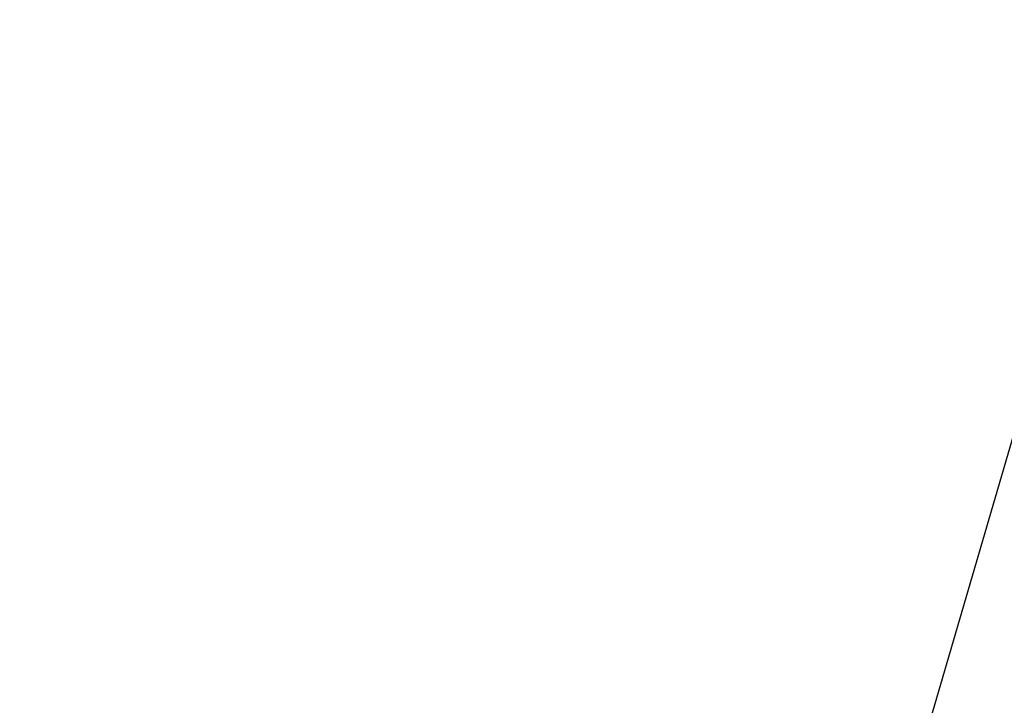
# Model space of a CAD drawing. Units: inches. Extents: x 3590 to 5167, y 65 to 1917.
# Tile 91 of 100: x 5052.5773 to 5052.8768, y 1788.8231 to 1789.0318. Entities that reach past the tile are written whole.
import ezdxf

# ---------------------------------------------------------------- set-up
doc = ezdxf.new("R2010")
doc.units = ezdxf.units.IN
for name, color, linetype, lineweight in [('A-ANNO-DIMS', 2, 'Continuous', 18), ('A-FLOR-PATT', 8, 'Continuous', 13), ('L-PLNT', 94, 'Continuous', 18)]:
    doc.layers.add(name, color=color, linetype=linetype, lineweight=lineweight)
doc.layers.add('DIENHOA', color=3, linetype='Continuous')
doc.styles.get("Standard").update_dxf_attribs({"font": 'arial.ttf'})
doc.dimstyles.new('ISO-25', dxfattribs={"dimtxt": 9, "dimasz": 2.5, "dimexe": 1.25, "dimexo": 0.625, "dimtad": 1, "dimdec": 1, "dimlunit": 3, "dimtxsty": 'Standard', "dimcen": 2.5, "dimadec": 0, "dimazin": 0, "dimtfac": 1, "dimtdec": 1, "dimtmove": 0, "dimatfit": 3, "dimfxl": 1, "dimarcsym": 0})

# ---------------------------------------------------------------- blocks, each defined once
blk = doc.blocks.new('Cay03_mb')
at = {"layer": 'DIENHOA'}
blk.add_line((118.956, 441.661), (96.72, 365.576), dxfattribs=at)
blk = doc.blocks.new('*D323')
at = {"layer": 'A-ANNO-DIMS', "color": 0, "lineweight": -2, "transparency": 16777216}
for p, q in [((5069.17227, 1795.21603), (5069.17227, 1874.95034)), ((5065.43703, 1795.21603), (5070.42227, 1795.21603)), ((5069.17227, 1769.30924), (5069.17227, 1792.71603)), ((5065.43703, 1766.80924), (5070.42227, 1766.80924))]:
    blk.add_line(p, q, dxfattribs=at)
at = {"layer": 'A-ANNO-DIMS', "color": 0, "transparency": 16777216}
for points in [[(5068.75561, 1792.71603), (5069.58894, 1792.71603), (5069.17227, 1795.21603)], [(5068.75561, 1769.30924), (5069.58894, 1769.30924), (5069.17227, 1766.80924)]]:
    blk.add_solid(points, dxfattribs=at)
at = {"layer": 'Defpoints', "color": 0, "transparency": 16777216}
for p in [(5064.81203, 1795.21603), (5069.17227, 1795.21603), (5064.81203, 1766.80924)]:
    blk.add_point(p, dxfattribs=at)
at = {"layer": 'A-ANNO-DIMS', "color": 0, "transparency": 16777216, "insert": (5063.89379, 1836.33318), "char_height": 9, "attachment_point": 5, "rotation": 90}
blk.add_mtext('2\'-4 1/2" TYP.', dxfattribs=at)

msp = doc.modelspace()

# ---------------------------------------------------------------- hatches: boundary and pattern name
at = {"layer": 'A-FLOR-PATT', "transparency": 33554687}
h = msp.add_hatch(dxfattribs=at)
h.set_pattern_fill('AR-HBONE', color=256, scale=0.2)
h.set_pattern_definition([(45, (-588.972, 0), (0, 28.73682), [60.96, -20.32]), (135, (-574.604, 14.368), (3e-15, 28.73682), [60.96, -20.32])])
h.paths.add_polyline_path([(5071.27403, 1796.99898), (4933.27403, 1796.99898), (4933.27403, 1753.99898), (4962.77403, 1753.99898, -0.414214), (4928.77403, 1719.99898), (4933.27403, 1718.99898), (4933.27403, 1334.99898), (5071.27403, 1334.99898)])
h.paths.add_polyline_path([(4951.78002, 1521.0767), (4951.7151, 1521.0404), (4951.56345, 1520.89532)], flags=16)
h.paths.add_polyline_path([(4952.267, 1521.37645), (4952.1977, 1521.37111), (4952.19823, 1521.35558)], flags=0)
h.paths.add_polyline_path([(4967.05076, 1529.72832), (4965.23122, 1528.69444), (4963.41109, 1527.71401), (4961.75649, 1526.85081), (4963.58887, 1527.44938), (4964.03555, 1527.47802), (4962.9755, 1527.24902), (4961.76022, 1526.85203), (4959.79219, 1525.83406), (4958.00498, 1524.89483), (4956.24031, 1523.92961), (4954.50395, 1522.91854), (4954.1294, 1522.68163), (4953.36051, 1521.99688), (4953.36558, 1521.99754), (4953.605, 1522.06367), (4955.10605, 1522.76083), (4956.92108, 1523.43405), (4958.67784, 1523.91513), (4960.35834, 1524.20036), (4961.94456, 1524.28606), (4964.17144, 1524.10849), (4965.95752, 1523.30903), (4963.86273, 1522.97565), (4965.18742, 1522.49898), (4963.36614, 1522.49715), (4961.54526, 1522.48682), (4959.76359, 1522.46077), (4958.30414, 1522.4188), (4957.97356, 1522.38829), (4956.30692, 1522.2324), (4954.71821, 1522.07143), (4953.25077, 1521.89915), (4953.52509, 1521.62277), (4954.33087, 1521.37883), (4956.24263, 1521.22987), (4958.03913, 1520.92952), (4959.68424, 1520.48339), (4961.16007, 1519.89569), (4963.10699, 1518.80022), (4964.39286, 1517.32518), (4962.97306, 1517.72596), (4964.55841, 1516.66059), (4965.40664, 1515.70779), (4963.50733, 1516.32179), (4961.67995, 1517.0051), (4959.93478, 1517.74489), (4958.2821, 1518.52833), (4956.73216, 1519.34257), (4955.29527, 1520.17478), (4954.67155, 1520.57237), (4954.51279, 1520.6271), (4955.65848, 1519.31837), (4956.70263, 1517.98232), (4957.64403, 1516.64663), (4958.48545, 1515.33439), (4959.54998, 1513.52398), (4960.43768, 1511.76936), (4958.84107, 1513.6196), (4957.45175, 1515.3249), (4955.8186, 1517.45855), (4956.66537, 1515.44764), (4957.11109, 1513.92292), (4957.44681, 1511.71434), (4957.07641, 1509.79288), (4956.53757, 1511.1103), (4955.99231, 1512.56892), (4955.44448, 1514.12509), (4954.89794, 1515.73518), (4954.35653, 1517.35553), (4953.82412, 1518.94251), (4953.30455, 1520.45247), (4953.06452, 1521.11563), (4952.97143, 1521.14607), (4952.94932, 1521.08646), (4952.72981, 1520.19905), (4953.3698, 1518.02364), (4953.75708, 1516.37279), (4954.05124, 1514.76538), (4954.26449, 1513.22121), (4954.47124, 1511.13121), (4954.4971, 1510.40174), (4954.40903, 1511.76006), (4954.26449, 1513.22121), (4954.05124, 1514.76538), (4953.75708, 1516.37279), (4953.3698, 1518.02364), (4952.87718, 1519.69813), (4952.7161, 1520.1412), (4952.53301, 1519.05871), (4952.37428, 1517.78881), (4952.21925, 1516.31167), (4952.04598, 1514.59986), (4951.83253, 1512.62598), (4951.55697, 1510.36259), (4951.20331, 1512.16818), (4950.85168, 1514.33931), (4950.98529, 1516.37594), (4951.6596, 1518.28625), (4952.59261, 1520.48085), (4952.35664, 1521.1299), (4951.85502, 1520.32753), (4950.83901, 1518.90828), (4949.77675, 1517.58658), (4948.91554, 1516.61731), (4948.11099, 1515.2561), (4947.0891, 1513.55389), (4945.88937, 1511.61495), (4946.32587, 1513.40232), (4946.5624, 1514.24913), (4945.52771, 1513.32668), (4944.58105, 1512.53126), (4946.01774, 1514.50825), (4947.2044, 1516.04763), (4947.89331, 1517.31331), (4949.30686, 1518.76446), (4950.41417, 1519.76716), (4950.45131, 1519.80628), (4952.267, 1521.37645), (4951.64457, 1521.49317), (4950.40371, 1521.17954), (4948.04447, 1520.35868), (4946.11863, 1519.45198), (4944.57182, 1518.47484), (4943.34962, 1517.44265), (4941.99695, 1515.91971), (4941.66146, 1515.27475), (4942.81332, 1516.98973), (4944.57182, 1518.47484), (4946.11863, 1519.45198), (4948.04447, 1520.35868), (4950.40371, 1521.17954), (4951.64457, 1521.49317), (4949.64678, 1521.86781), (4948.59979, 1521.75633), (4947.12629, 1521.5699), (4945.42015, 1521.34763), (4943.44969, 1521.10462), (4941.18319, 1520.85596), (4942.86028, 1521.61265), (4943.87308, 1522.03014), (4942.95216, 1521.9093), (4941.40968, 1521.48512), (4939.54287, 1520.67019), (4938.96775, 1520.2255), (4940.73284, 1521.29899), (4942.95216, 1521.9093), (4943.70184, 1522.00767), (4945.89419, 1522.69998), (4947.56488, 1522.71399), (4948.92086, 1522.56573), (4951.13144, 1522.18271), (4950.97062, 1522.2969), (4948.12924, 1523.00563), (4946.03496, 1523.70671), (4944.23235, 1524.52143), (4942.70692, 1525.46111), (4941.44419, 1526.53707), (4940.42968, 1527.76062), (4939.6489, 1529.14306), (4941.42091, 1528.12232), (4943.14742, 1527.13248), (4944.84093, 1526.17457), (4946.51394, 1525.24959), (4948.17893, 1524.35855), (4948.36457, 1524.26336), (4946.47531, 1526.04459), (4945.18083, 1527.54042), (4944.19039, 1529.03339), (4943.49559, 1530.53985), (4943.27808, 1531.3597), (4942.49849, 1531.91903), (4943.11353, 1531.76249), (4942.95927, 1533.6586), (4944.13953, 1531.9886), (4944.61171, 1531.32339), (4946.20163, 1530.46341), (4947.48567, 1529.50925), (4948.79027, 1528.22649), (4950.36754, 1526.23746), (4949.48547, 1528.15549), (4948.85128, 1530.12254), (4948.49054, 1532.04127), (4948.38105, 1533.91822), (4948.50062, 1535.7599), (4948.82704, 1537.57284), (4949.41803, 1535.56526), (4949.95684, 1533.56932), (4950.46414, 1531.5861), (4950.96058, 1529.6167), (4951.3911, 1527.95448), (4951.72352, 1530.68689), (4952.20106, 1532.57994), (4952.88914, 1534.32964), (4953.77035, 1535.95123), (4954.82726, 1537.45995), (4954.52145, 1535.38966), (4954.27314, 1533.93684), (4955.57999, 1535.6627), (4956.74758, 1536.73859), (4956.15852, 1534.78029), (4955.58917, 1532.87334), (4955.04336, 1531.00581), (4954.52493, 1529.16576), (4954.03771, 1527.34127), (4953.63833, 1525.73298), (4953.61143, 1525.58564), (4953.39805, 1524.16565), (4953.38219, 1524.00887), (4954.06955, 1525.47563), (4954.91212, 1527.02173), (4956.13627, 1528.89351), (4957.84668, 1530.57701), (4959.37601, 1531.54014), (4958.25596, 1530.10398), (4957.14284, 1528.66291), (4956.06626, 1527.24305), (4955.05579, 1525.87054), (4954.14104, 1524.57149), (4953.35159, 1523.37204), (4953.31079, 1523.30299), (4953.27253, 1522.92478), (4953.26102, 1522.38213), (4954.1031, 1523.37273), (4954.63005, 1524.28376), (4955.96149, 1526.35767), (4957.23002, 1528.12969), (4958.42057, 1529.60864), (4960.03671, 1531.36792), (4961.3736, 1532.3752), (4962.1015, 1532.77), (4961.06994, 1531.06113), (4959.98733, 1529.43811), (4958.86851, 1527.90803), (4958.15046, 1527.00742), (4959.80291, 1528.00314), (4961.58854, 1528.79257), (4963.39087, 1529.32783), (4965.21118, 1529.63205)], flags=16)
h.paths.add_polyline_path([(4962.94387, 1523.18187), (4961.10714, 1523.42192), (4960.39205, 1523.36158), (4962.34964, 1523.33061)], flags=0)
h.paths.add_polyline_path([(5049.54129, 1584.55089), (5049.47636, 1584.51458), (5049.32471, 1584.3695)], flags=16)
h.paths.add_polyline_path([(5050.02827, 1584.85063), (5049.95897, 1584.84529), (5049.95949, 1584.82976)], flags=0)
h.paths.add_polyline_path([(5042.33308, 1581.94902), (5043.8799, 1582.92616), (5045.80573, 1583.83286), (5048.16498, 1584.65372), (5049.40583, 1584.96736), (5047.40804, 1585.34199), (5046.36106, 1585.23052), (5044.88755, 1585.04408), (5043.18142, 1584.82181), (5041.21095, 1584.5788), (5038.94446, 1584.33014), (5040.62155, 1585.08683), (5041.63434, 1585.50432), (5040.71343, 1585.38348), (5039.17095, 1584.9593), (5037.30414, 1584.14438), (5036.72901, 1583.69969), (5038.4941, 1584.77317), (5040.71343, 1585.38348), (5041.4631, 1585.48185), (5043.65545, 1586.17416), (5045.32615, 1586.18818), (5046.68212, 1586.03992), (5048.8927, 1585.6569), (5048.73188, 1585.77108), (5045.89051, 1586.47981), (5043.79622, 1587.18089), (5041.99361, 1587.99561), (5040.46818, 1588.9353), (5039.20546, 1590.01125), (5038.19095, 1591.2348), (5037.41016, 1592.61725), (5039.18217, 1591.5965), (5040.90868, 1590.60667), (5042.6022, 1589.64876), (5044.2752, 1588.72378), (5045.94019, 1587.83274), (5046.12584, 1587.73754), (5044.23658, 1589.51878), (5042.9421, 1591.01461), (5041.95166, 1592.50757), (5041.25685, 1594.01403), (5041.03935, 1594.83388), (5040.25976, 1595.39321), (5040.8748, 1595.23667), (5040.72054, 1597.13279), (5041.9008, 1595.46278), (5042.37297, 1594.79758), (5043.96289, 1593.93759), (5045.24694, 1592.98344), (5046.55153, 1591.70068), (5048.12881, 1589.71164), (5047.24673, 1591.62967), (5046.61254, 1593.59672), (5046.2518, 1595.51546), (5046.14232, 1597.3924), (5046.26189, 1599.23408), (5046.5883, 1601.04703), (5047.17929, 1599.03944), (5047.71811, 1597.0435), (5048.22541, 1595.06028), (5048.72184, 1593.09089), (5049.15237, 1591.42866), (5049.48478, 1594.16107), (5049.96233, 1596.05412), (5050.65041, 1597.80382), (5051.53161, 1599.42541), (5052.58852, 1600.93414), (5052.28271, 1598.86384), (5052.03441, 1597.41102), (5053.34126, 1599.13689), (5054.50884, 1600.21277), (5053.91979, 1598.25447), (5053.35044, 1596.34752), (5052.80463, 1594.47999), (5052.2862, 1592.63995), (5051.79898, 1590.81546), (5051.39959, 1589.20716), (5051.3727, 1589.05983), (5051.15931, 1587.63984), (5051.14346, 1587.48305), (5051.83082, 1588.94982), (5052.67339, 1590.49592), (5053.89754, 1592.3677), (5055.60794, 1594.05119), (5057.13728, 1595.01432), (5056.01722, 1593.57817), (5054.90411, 1592.1371), (5053.82752, 1590.71724), (5052.81705, 1589.34472), (5051.9023, 1588.04567), (5051.11286, 1586.84622), (5051.07205, 1586.77718), (5051.03379, 1586.39896), (5051.02228, 1585.85631), (5051.86437, 1586.84692), (5052.39131, 1587.75794), (5053.72275, 1589.83185), (5054.99128, 1591.60387), (5056.18183, 1593.08282), (5057.79798, 1594.84211), (5059.13486, 1595.84938), (5059.86276, 1596.24419), (5058.83121, 1594.53531), (5057.7486, 1592.9123), (5056.62978, 1591.38221), (5055.91173, 1590.4816), (5057.56418, 1591.47732), (5059.34981, 1592.26675), (5061.15214, 1592.80202), (5062.97245, 1593.10624), (5064.81203, 1593.20251), (5062.99248, 1592.16863), (5061.17235, 1591.18819), (5059.51775, 1590.325), (5061.35014, 1590.92356), (5061.79682, 1590.95221), (5060.73676, 1590.7232), (5059.52148, 1590.32622), (5057.55345, 1589.30825), (5055.76625, 1588.36901), (5054.00157, 1587.40379), (5052.26521, 1586.39273), (5051.89067, 1586.15581), (5051.12177, 1585.47106), (5051.12684, 1585.47172), (5051.36627, 1585.53786), (5052.86732, 1586.23502), (5054.68234, 1586.90824), (5056.4391, 1587.38931), (5058.1196, 1587.67454), (5059.70582, 1587.76024), (5061.93271, 1587.58268), (5063.71878, 1586.78321), (5061.62399, 1586.44983), (5062.94869, 1585.97317), (5061.12741, 1585.97133), (5059.30653, 1585.961), (5057.52486, 1585.93496), (5056.06541, 1585.89299), (5055.73482, 1585.86247), (5054.06819, 1585.70658), (5052.47947, 1585.54561), (5051.01204, 1585.37333), (5051.28635, 1585.09695), (5052.09214, 1584.85301), (5054.00389, 1584.70406), (5055.8004, 1584.4037), (5057.44551, 1583.95757), (5058.92133, 1583.36987), (5060.86825, 1582.27441), (5062.15413, 1580.79937), (5060.73433, 1581.20015), (5062.31967, 1580.13477), (5063.1679, 1579.18198), (5061.2686, 1579.79597), (5059.44122, 1580.47928), (5057.69605, 1581.21908), (5056.04336, 1582.00251), (5054.49343, 1582.81675), (5053.05653, 1583.64897), (5052.43281, 1584.04656), (5052.27405, 1584.10128), (5053.41974, 1582.79255), (5054.4639, 1581.4565), (5055.40529, 1580.12081), (5056.24672, 1578.80858), (5057.31125, 1576.99816), (5058.19895, 1575.24354), (5056.60234, 1577.09378), (5055.21301, 1578.79908), (5053.57987, 1580.93274), (5054.42664, 1578.92183), (5054.87235, 1577.3971), (5055.20808, 1575.18852), (5054.83767, 1573.26706), (5054.29883, 1574.58448), (5053.75357, 1576.0431), (5053.20575, 1577.59927), (5052.6592, 1579.20936), (5052.1178, 1580.82971), (5051.58538, 1582.41669), (5051.06582, 1583.92666), (5050.82578, 1584.58981), (5050.7327, 1584.62025), (5050.71058, 1584.56064), (5050.49108, 1583.67323), (5051.13107, 1581.49782), (5051.51835, 1579.84698), (5051.8125, 1578.23957), (5052.02575, 1576.69539), (5052.23251, 1574.6054), (5052.25836, 1573.87593), (5052.1703, 1575.23424), (5052.02575, 1576.69539), (5051.8125, 1578.23957), (5051.51835, 1579.84698), (5051.13107, 1581.49782), (5050.63844, 1583.17231), (5050.47736, 1583.61538), (5050.29428, 1582.53289), (5050.13554, 1581.26299), (5049.98051, 1579.78585), (5049.80724, 1578.07405), (5049.59379, 1576.10016), (5049.31823, 1573.83678), (5048.96458, 1575.64237), (5048.61294, 1577.8135), (5048.74656, 1579.85012), (5049.42086, 1581.76043), (5050.35388, 1583.95503), (5050.1179, 1584.60408), (5049.61629, 1583.80172), (5048.60027, 1582.38246), (5047.53801, 1581.06076), (5046.67681, 1580.09149), (5045.87225, 1578.73029), (5044.85036, 1577.02808), (5043.65063, 1575.08913), (5044.08713, 1576.8765), (5044.32366, 1577.72331), (5043.28898, 1576.80086), (5042.34232, 1576.00545), (5043.779, 1577.98243), (5044.96566, 1579.52182), (5045.65457, 1580.78749), (5047.06813, 1582.23865), (5048.17543, 1583.24134), (5048.21258, 1583.28047), (5050.02827, 1584.85063), (5049.40583, 1584.96736), (5048.16498, 1584.65372), (5045.80573, 1583.83286), (5043.8799, 1582.92616), (5042.33308, 1581.94902), (5041.11088, 1580.91684), (5039.75821, 1579.39389), (5039.42272, 1578.74894), (5040.57458, 1580.46391)], flags=16)
h.paths.add_polyline_path([(4954.79872, 1533.12029), (4954.26249, 1532.07935), (4953.83112, 1530.93464), (4953.50472, 1529.63602), (4953.28338, 1528.13331), (4953.16721, 1526.37637), (4953.15631, 1524.31504), (4953.27669, 1521.23629), (4952.80168, 1521.84177), (4951.55695, 1521.99789), (4950.97575, 1521.9613), (4952.66059, 1521.94097), (4952.80168, 1521.84177), (4953.15249, 1523.59258), (4953.16721, 1526.37637), (4953.28338, 1528.13331), (4953.60929, 1530.34598), (4954.45558, 1532.59174)], flags=0)
h.paths.add_polyline_path([(5050.56294, 1585.31596), (5049.31822, 1585.47208), (5048.73702, 1585.43548), (5050.42186, 1585.41516), (5050.56294, 1585.31596), (5050.91375, 1587.06676), (5050.92848, 1589.85056), (5051.04465, 1591.6075), (5051.37055, 1593.82017), (5052.21684, 1596.06593), (5052.55999, 1596.59447), (5052.02375, 1595.55353), (5051.59238, 1594.40883), (5051.26598, 1593.1102), (5051.04465, 1591.6075), (5050.92848, 1589.85056), (5050.91757, 1587.78922), (5051.03795, 1584.71048)], flags=0)
h.paths.add_polyline_path([(5058.15332, 1586.83576), (5060.11091, 1586.80479), (5060.70514, 1586.65605), (5058.8684, 1586.8961)], flags=0)
h.paths.add_polyline_path([(5049.54129, 1430.93611), (5049.47636, 1430.8998), (5049.32471, 1430.75472)], flags=16)
h.paths.add_polyline_path([(5050.02827, 1431.23585), (5049.95897, 1431.23051), (5049.95949, 1431.21498)], flags=0)
h.paths.add_polyline_path([(5046.5883, 1447.43225), (5047.17929, 1445.42467), (5047.71811, 1443.42872), (5048.22541, 1441.4455), (5048.72184, 1439.47611), (5049.15237, 1437.81388), (5049.48478, 1440.5463), (5049.96233, 1442.43934), (5050.65041, 1444.18904), (5051.53161, 1445.81063), (5052.58852, 1447.31936), (5052.28271, 1445.24906), (5052.03441, 1443.79624), (5053.34126, 1445.52211), (5054.50884, 1446.59799), (5053.91979, 1444.63969), (5053.35044, 1442.73274), (5052.80463, 1440.86521), (5052.2862, 1439.02517), (5051.79898, 1437.20068), (5051.39959, 1435.59238), (5051.3727, 1435.44505), (5051.15931, 1434.02506), (5051.14346, 1433.86828), (5051.83082, 1435.33504), (5052.67339, 1436.88114), (5053.89754, 1438.75292), (5055.60794, 1440.43641), (5057.13728, 1441.39954), (5056.01722, 1439.96339), (5054.90411, 1438.52232), (5053.82752, 1437.10246), (5052.81705, 1435.72994), (5051.9023, 1434.4309), (5051.11286, 1433.23145), (5051.07205, 1433.1624), (5051.03379, 1432.78418), (5051.02228, 1432.24153), (5051.86437, 1433.23214), (5052.39131, 1434.14316), (5053.72275, 1436.21707), (5054.99128, 1437.98909), (5056.18183, 1439.46805), (5057.79798, 1441.22733), (5059.13486, 1442.23461), (5059.86276, 1442.62941), (5058.83121, 1440.92053), (5057.7486, 1439.29752), (5056.62978, 1437.76743), (5055.91173, 1436.86682), (5057.56418, 1437.86255), (5059.34981, 1438.65197), (5061.15214, 1439.18724), (5062.97245, 1439.49146), (5064.81203, 1439.58773), (5062.99248, 1438.55385), (5061.17235, 1437.57342), (5059.51775, 1436.71022), (5061.35014, 1437.30879), (5061.79682, 1437.33743), (5060.73676, 1437.10842), (5059.52148, 1436.71144), (5057.55345, 1435.69347), (5055.76625, 1434.75423), (5054.00157, 1433.78901), (5052.26521, 1432.77795), (5051.89067, 1432.54103), (5051.12177, 1431.85628), (5051.12684, 1431.85694), (5051.36627, 1431.92308), (5052.86732, 1432.62024), (5054.68234, 1433.29346), (5056.4391, 1433.77453), (5058.1196, 1434.05976), (5059.70582, 1434.14546), (5061.93271, 1433.9679), (5063.71878, 1433.16843), (5061.62399, 1432.83505), (5062.94869, 1432.35839), (5061.12741, 1432.35655), (5059.30653, 1432.34623), (5057.52486, 1432.32018), (5056.06541, 1432.27821), (5055.73482, 1432.24769), (5054.06819, 1432.09181), (5052.47947, 1431.93083), (5051.01204, 1431.75856), (5051.28635, 1431.48218), (5052.09214, 1431.23823), (5054.00389, 1431.08928), (5055.8004, 1430.78892), (5057.44551, 1430.34279), (5058.92133, 1429.75509), (5060.86825, 1428.65963), (5062.15413, 1427.18459), (5060.73433, 1427.58537), (5062.31967, 1426.52), (5063.1679, 1425.5672), (5061.2686, 1426.18119), (5059.44122, 1426.86451), (5057.69605, 1427.6043), (5056.04336, 1428.38773), (5054.49343, 1429.20197), (5053.05653, 1430.03419), (5052.43281, 1430.43178), (5052.27405, 1430.48651), (5053.41974, 1429.17777), (5054.4639, 1427.84172), (5055.40529, 1426.50603), (5056.24672, 1425.1938), (5057.31125, 1423.38338), (5058.19895, 1421.62877), (5056.60234, 1423.479), (5055.21301, 1425.1843), (5053.57987, 1427.31796), (5054.42664, 1425.30705), (5054.87235, 1423.78233), (5055.20808, 1421.57374), (5054.83767, 1419.65228), (5054.29883, 1420.9697), (5053.75357, 1422.42832), (5053.20575, 1423.9845), (5052.6592, 1425.59458), (5052.1178, 1427.21493), (5051.58538, 1428.80191), (5051.06582, 1430.31188), (5050.82578, 1430.97503), (5050.7327, 1431.00547), (5050.71058, 1430.94586), (5050.49108, 1430.05845), (5051.13107, 1427.88305), (5051.51835, 1426.2322), (5051.8125, 1424.62479), (5052.02575, 1423.08061), (5052.23251, 1420.99062), (5052.25836, 1420.26115), (5052.1703, 1421.61947), (5052.02575, 1423.08061), (5051.8125, 1424.62479), (5051.51835, 1426.2322), (5051.13107, 1427.88305), (5050.63844, 1429.55753), (5050.47736, 1430.0006), (5050.29428, 1428.91811), (5050.13554, 1427.64821), (5049.98051, 1426.17107), (5049.80724, 1424.45927), (5049.59379, 1422.48539), (5049.31823, 1420.222), (5048.96458, 1422.02759), (5048.61294, 1424.19872), (5048.74656, 1426.23534), (5049.42086, 1428.14565), (5050.35388, 1430.34025), (5050.1179, 1430.98931), (5049.61629, 1430.18694), (5048.60027, 1428.76768), (5047.53801, 1427.44598), (5046.67681, 1426.47671), (5045.87225, 1425.11551), (5044.85036, 1423.4133), (5043.65063, 1421.47435), (5044.08713, 1423.26172), (5044.32366, 1424.10854), (5043.28898, 1423.18608), (5042.34232, 1422.39067), (5043.779, 1424.36765), (5044.96566, 1425.90704), (5045.65457, 1427.17272), (5047.06813, 1428.62387), (5048.17543, 1429.62657), (5048.21258, 1429.66569), (5050.02827, 1431.23585), (5049.40583, 1431.35258), (5048.16498, 1431.03894), (5045.80573, 1430.21809), (5043.8799, 1429.31139), (5042.33308, 1428.33424), (5041.11088, 1427.30206), (5039.75821, 1425.77911), (5039.42272, 1425.13416), (5040.57458, 1426.84914), (5042.33308, 1428.33424), (5043.8799, 1429.31139), (5045.80573, 1430.21809), (5048.16498, 1431.03894), (5049.40583, 1431.35258), (5047.40804, 1431.72722), (5046.36106, 1431.61574), (5044.88755, 1431.42931), (5043.18142, 1431.20704), (5041.21095, 1430.96402), (5038.94446, 1430.71536), (5040.62155, 1431.47205), (5041.63434, 1431.88954), (5040.71343, 1431.76871), (5039.17095, 1431.34453), (5037.30414, 1430.5296), (5036.72901, 1430.08491), (5038.4941, 1431.1584), (5040.71343, 1431.76871), (5041.4631, 1431.86707), (5043.65545, 1432.55939), (5045.32615, 1432.5734), (5046.68212, 1432.42514), (5048.8927, 1432.04212), (5048.73188, 1432.1563), (5045.89051, 1432.86503), (5043.79622, 1433.56611), (5041.99361, 1434.38083), (5040.46818, 1435.32052), (5039.20546, 1436.39648), (5038.19095, 1437.62002), (5037.41016, 1439.00247), (5039.18217, 1437.98172), (5040.90868, 1436.99189), (5042.6022, 1436.03398), (5044.2752, 1435.109), (5045.94019, 1434.21796), (5046.12584, 1434.12276), (5044.23658, 1435.904), (5042.9421, 1437.39983), (5041.95166, 1438.8928), (5041.25685, 1440.39925), (5041.03935, 1441.2191), (5040.25976, 1441.77844), (5040.8748, 1441.62189), (5040.72054, 1443.51801), (5041.9008, 1441.848), (5042.37297, 1441.1828), (5043.96289, 1440.32282), (5045.24694, 1439.36866), (5046.55153, 1438.0859), (5048.12881, 1436.09686), (5047.24673, 1438.01489), (5046.61254, 1439.98195), (5046.2518, 1441.90068), (5046.14232, 1443.77762), (5046.26189, 1445.6193)], flags=16)
h.paths.add_polyline_path([(5052.38176, 1444.25496), (5051.62263, 1442.77987), (5052.02375, 1441.93875), (5052.55999, 1442.9797)], flags=0)
h.paths.add_polyline_path([(5050.56294, 1431.70118), (5049.31822, 1431.8573), (5048.73702, 1431.82071), (5050.42186, 1431.80038)], flags=0)
h.paths.add_polyline_path([(5058.15332, 1433.22098), (5060.11091, 1433.19001), (5060.70514, 1433.04127), (5058.8684, 1433.28132)], flags=0)
h.paths.add_polyline_path([(5049.54129, 1352.28535), (5049.47636, 1352.24904), (5049.32471, 1352.10396)], flags=16)
h.paths.add_polyline_path([(5050.02827, 1352.58509), (5049.95897, 1352.57975), (5049.95949, 1352.56422)], flags=0)
h.paths.add_polyline_path([(5046.5883, 1368.78149), (5047.17929, 1366.7739), (5047.71811, 1364.77796), (5048.22541, 1362.79474), (5048.72184, 1360.82534), (5049.15237, 1359.16312), (5049.48478, 1361.89553), (5049.96233, 1363.78858), (5050.65041, 1365.53828), (5051.53161, 1367.15987), (5052.58852, 1368.6686), (5052.28271, 1366.5983), (5052.03441, 1365.14548), (5053.34126, 1366.87135), (5054.50884, 1367.94723), (5053.91979, 1365.98893), (5053.35044, 1364.08198), (5052.80463, 1362.21445), (5052.2862, 1360.37441), (5051.79898, 1358.54992), (5051.39959, 1356.94162), (5051.3727, 1356.79428), (5051.15931, 1355.37429), (5051.14346, 1355.21751), (5051.83082, 1356.68428), (5052.67339, 1358.23037), (5053.89754, 1360.10216), (5055.60794, 1361.78565), (5057.13728, 1362.74878), (5056.01722, 1361.31262), (5054.90411, 1359.87155), (5053.82752, 1358.4517), (5052.81705, 1357.07918), (5051.9023, 1355.78013), (5051.11286, 1354.58068), (5051.07205, 1354.51164), (5051.03379, 1354.13342), (5051.02228, 1353.59077), (5051.86437, 1354.58137), (5052.39131, 1355.4924), (5053.72275, 1357.56631), (5054.99128, 1359.33833), (5056.18183, 1360.81728), (5057.79798, 1362.57656), (5059.13486, 1363.58384), (5059.86276, 1363.97864), (5058.83121, 1362.26977), (5057.7486, 1360.64675), (5056.62978, 1359.11667), (5055.91173, 1358.21606), (5057.56418, 1359.21178), (5059.34981, 1360.00121), (5061.15214, 1360.53648), (5062.97245, 1360.84069), (5064.81203, 1360.93697), (5062.99248, 1359.90308), (5061.17235, 1358.92265), (5059.51775, 1358.05946), (5061.35014, 1358.65802), (5061.79682, 1358.68666), (5060.73676, 1358.45766), (5059.52148, 1358.06068), (5057.55345, 1357.0427), (5055.76625, 1356.10347), (5054.00157, 1355.13825), (5052.26521, 1354.12718), (5051.89067, 1353.89027), (5051.12177, 1353.20552), (5051.12684, 1353.20618), (5051.36627, 1353.27231), (5052.86732, 1353.96947), (5054.68234, 1354.6427), (5056.4391, 1355.12377), (5058.1196, 1355.409), (5059.70582, 1355.4947), (5061.93271, 1355.31713), (5063.71878, 1354.51767), (5061.62399, 1354.18429), (5062.94869, 1353.70763), (5061.12741, 1353.70579), (5059.30653, 1353.69546), (5057.52486, 1353.66942), (5056.06541, 1353.62744), (5055.73482, 1353.59693), (5054.06819, 1353.44104), (5052.47947, 1353.28007), (5051.01204, 1353.10779), (5051.28635, 1352.83141), (5052.09214, 1352.58747), (5054.00389, 1352.43852), (5055.8004, 1352.13816), (5057.44551, 1351.69203), (5058.92133, 1351.10433), (5060.86825, 1350.00887), (5062.15413, 1348.53382), (5060.73433, 1348.9346), (5062.31967, 1347.86923), (5063.1679, 1346.91643), (5061.2686, 1347.53043), (5059.44122, 1348.21374), (5057.69605, 1348.95353), (5056.04336, 1349.73697), (5054.49343, 1350.55121), (5053.05653, 1351.38342), (5052.43281, 1351.78101), (5052.27405, 1351.83574), (5053.41974, 1350.52701), (5054.4639, 1349.19096), (5055.40529, 1347.85527), (5056.24672, 1346.54303), (5057.31125, 1344.73262), (5058.19895, 1342.978), (5056.60234, 1344.82824), (5055.21301, 1346.53354), (5053.57987, 1348.6672), (5054.42664, 1346.65629), (5054.87235, 1345.13156), (5055.20808, 1342.92298), (5054.83767, 1341.00152), (5054.29883, 1342.31894), (5053.75357, 1343.77756), (5053.20575, 1345.33373), (5052.6592, 1346.94382), (5052.1178, 1348.56417), (5051.58538, 1350.15115), (5051.06582, 1351.66111), (5050.82578, 1352.32427), (5050.7327, 1352.35471), (5050.71058, 1352.2951), (5050.49108, 1351.40769), (5051.13107, 1349.23228), (5051.51835, 1347.58144), (5051.8125, 1345.97403), (5052.02575, 1344.42985), (5052.23251, 1342.33986), (5052.25836, 1341.61039), (5052.1703, 1342.9687), (5052.02575, 1344.42985), (5051.8125, 1345.97403), (5051.51835, 1347.58144), (5051.13107, 1349.23228), (5050.63844, 1350.90677), (5050.47736, 1351.34984), (5050.29428, 1350.26735), (5050.13554, 1348.99745), (5049.98051, 1347.52031), (5049.80724, 1345.80851), (5049.59379, 1343.83462), (5049.31823, 1341.57124), (5048.96458, 1343.37683), (5048.61294, 1345.54796), (5048.74656, 1347.58458), (5049.42086, 1349.49489), (5050.35388, 1351.68949), (5050.1179, 1352.33854), (5049.61629, 1351.53617), (5048.60027, 1350.11692), (5047.53801, 1348.79522), (5046.67681, 1347.82595), (5045.87225, 1346.46475), (5044.85036, 1344.76253), (5043.65063, 1342.82359), (5044.08713, 1344.61096), (5044.32366, 1345.45777), (5043.28898, 1344.53532), (5042.34232, 1343.7399), (5043.779, 1345.71689), (5044.96566, 1347.25627), (5045.65457, 1348.52195), (5047.06813, 1349.9731), (5048.17543, 1350.9758), (5048.21258, 1351.01493), (5050.02827, 1352.58509), (5049.40583, 1352.70181), (5048.16498, 1352.38818), (5045.80573, 1351.56732), (5043.8799, 1350.66062), (5042.33308, 1349.68348), (5041.11088, 1348.65129), (5039.75821, 1347.12835), (5039.42272, 1346.4834), (5040.57458, 1348.19837), (5042.33308, 1349.68348), (5043.8799, 1350.66062), (5045.80573, 1351.56732), (5048.16498, 1352.38818), (5049.40583, 1352.70181), (5047.40804, 1353.07645), (5046.36106, 1352.96498), (5044.88755, 1352.77854), (5043.18142, 1352.55627), (5041.21095, 1352.31326), (5038.94446, 1352.0646), (5040.62155, 1352.82129), (5041.63434, 1353.23878), (5040.71343, 1353.11794), (5039.17095, 1352.69376), (5037.30414, 1351.87884), (5036.72901, 1351.43415), (5038.4941, 1352.50763), (5040.71343, 1353.11794), (5041.4631, 1353.21631), (5043.65545, 1353.90862), (5045.32615, 1353.92263), (5046.68212, 1353.77438), (5048.8927, 1353.39136), (5048.73188, 1353.50554), (5045.89051, 1354.21427), (5043.79622, 1354.91535), (5041.99361, 1355.73007), (5040.46818, 1356.66975), (5039.20546, 1357.74571), (5038.19095, 1358.96926), (5037.41016, 1360.35171), (5039.18217, 1359.33096), (5040.90868, 1358.34112), (5042.6022, 1357.38321), (5044.2752, 1356.45824), (5045.94019, 1355.5672), (5046.12584, 1355.472), (5044.23658, 1357.25323), (5042.9421, 1358.74906), (5041.95166, 1360.24203), (5041.25685, 1361.74849), (5041.03935, 1362.56834), (5040.25976, 1363.12767), (5040.8748, 1362.97113), (5040.72054, 1364.86725), (5041.9008, 1363.19724), (5042.37297, 1362.53203), (5043.96289, 1361.67205), (5045.24694, 1360.7179), (5046.55153, 1359.43513), (5048.12881, 1357.4461), (5047.24673, 1359.36413), (5046.61254, 1361.33118), (5046.2518, 1363.24992), (5046.14232, 1365.12686), (5046.26189, 1366.96854)], flags=16)
h.paths.add_polyline_path([(5052.38176, 1365.6042), (5051.62263, 1364.12911), (5052.02375, 1363.28799), (5052.55999, 1364.32893)], flags=0)
h.paths.add_polyline_path([(4951.78002, 1698.04081), (4951.7151, 1698.0045), (4951.56345, 1697.85942)], flags=16)
h.paths.add_polyline_path([(4952.267, 1698.34055), (4952.1977, 1698.33521), (4952.19823, 1698.31968)], flags=0)
h.paths.add_polyline_path([(4957.07641, 1686.75698), (4956.53757, 1688.0744), (4955.99231, 1689.53302), (4955.44448, 1691.08919), (4954.89794, 1692.69928), (4954.35653, 1694.31963), (4953.82412, 1695.90661), (4953.30455, 1697.41658), (4953.06452, 1698.07973), (4952.97143, 1698.11017), (4952.94932, 1698.05056), (4952.72981, 1697.16315), (4953.3698, 1694.98774), (4953.75708, 1693.3369), (4954.05124, 1691.72949), (4954.26449, 1690.18531), (4954.47124, 1688.09532), (4954.4971, 1687.36585), (4954.40903, 1688.72416), (4954.26449, 1690.18531), (4954.05124, 1691.72949), (4953.75708, 1693.3369), (4953.3698, 1694.98774), (4952.87718, 1696.66223), (4952.7161, 1697.1053), (4952.53301, 1696.02281), (4952.37428, 1694.75291), (4952.21925, 1693.27577), (4952.04598, 1691.56397), (4951.83253, 1689.59008), (4951.55697, 1687.3267), (4951.20331, 1689.13229), (4950.85168, 1691.30342), (4950.98529, 1693.34004), (4951.6596, 1695.25035), (4952.59261, 1697.44495), (4952.35664, 1698.09401), (4951.85502, 1697.29164), (4950.83901, 1695.87238), (4949.77675, 1694.55068), (4948.91554, 1693.58141), (4948.11099, 1692.22021), (4947.0891, 1690.518), (4945.88937, 1688.57905), (4946.32587, 1690.36642), (4946.5624, 1691.21323), (4945.52771, 1690.29078), (4944.58105, 1689.49537), (4946.01774, 1691.47235), (4947.2044, 1693.01174), (4947.89331, 1694.27741), (4949.30686, 1695.72857), (4950.41417, 1696.73127), (4950.45131, 1696.77039), (4952.267, 1698.34055), (4951.64457, 1698.45728), (4950.40371, 1698.14364), (4948.04447, 1697.32278), (4946.11863, 1696.41608), (4944.57182, 1695.43894), (4943.34962, 1694.40676), (4941.99695, 1692.88381), (4941.66146, 1692.23886), (4942.81332, 1693.95383), (4944.57182, 1695.43894), (4946.11863, 1696.41608), (4948.04447, 1697.32278), (4950.40371, 1698.14364), (4951.64457, 1698.45728), (4949.64678, 1698.83191), (4948.59979, 1698.72044), (4947.12629, 1698.53401), (4945.42015, 1698.31174), (4943.44969, 1698.06872), (4941.18319, 1697.82006), (4942.86028, 1698.57675), (4943.87308, 1698.99424), (4942.95216, 1698.8734), (4941.40968, 1698.44922), (4939.54287, 1697.6343), (4938.96775, 1697.18961), (4940.73284, 1698.26309), (4942.95216, 1698.8734), (4943.70184, 1698.97177), (4945.89419, 1699.66409), (4947.56488, 1699.6781), (4948.92086, 1699.52984), (4951.13144, 1699.14682), (4950.97062, 1699.261), (4948.12924, 1699.96973), (4946.03496, 1700.67081), (4944.23235, 1701.48553), (4942.70692, 1702.42522), (4941.44419, 1703.50117), (4940.42968, 1704.72472), (4939.6489, 1706.10717), (4941.42091, 1705.08642), (4943.14742, 1704.09659), (4944.84093, 1703.13868), (4946.51394, 1702.2137), (4948.17893, 1701.32266), (4948.36457, 1701.22746), (4946.47531, 1703.0087), (4945.18083, 1704.50453), (4944.19039, 1705.9975), (4943.49559, 1707.50395), (4943.27808, 1708.3238), (4942.49849, 1708.88314), (4943.11353, 1708.72659), (4942.95927, 1710.62271), (4944.13953, 1708.9527), (4944.61171, 1708.2875), (4946.20163, 1707.42751), (4947.48567, 1706.47336), (4948.79027, 1705.1906), (4950.36754, 1703.20156), (4949.48547, 1705.11959), (4948.85128, 1707.08664), (4948.49054, 1709.00538), (4948.38105, 1710.88232), (4948.50062, 1712.724), (4948.82704, 1714.53695), (4949.41803, 1712.52937), (4949.95684, 1710.53342), (4950.46414, 1708.5502), (4950.96058, 1706.58081), (4951.3911, 1704.91858), (4951.72352, 1707.65099), (4952.20106, 1709.54404), (4952.88914, 1711.29374), (4953.77035, 1712.91533), (4954.82726, 1714.42406), (4954.52145, 1712.35376), (4954.27314, 1710.90094), (4955.57999, 1712.62681), (4956.74758, 1713.70269), (4956.15852, 1711.74439), (4955.58917, 1709.83744), (4955.04336, 1707.96991), (4954.52493, 1706.12987), (4954.03771, 1704.30538), (4953.63833, 1702.69708), (4953.61143, 1702.54975), (4953.39805, 1701.12976), (4953.38219, 1700.97297), (4954.06955, 1702.43974), (4954.91212, 1703.98584), (4956.13627, 1705.85762), (4957.84668, 1707.54111), (4959.37601, 1708.50424), (4958.25596, 1707.06809), (4957.14284, 1705.62702), (4956.06626, 1704.20716), (4955.05579, 1702.83464), (4954.14104, 1701.53559), (4953.35159, 1700.33614), (4953.31079, 1700.2671), (4953.27253, 1699.88888), (4953.26102, 1699.34623), (4954.1031, 1700.33684), (4954.63005, 1701.24786), (4955.96149, 1703.32177), (4957.23002, 1705.09379), (4958.42057, 1706.57274), (4960.03671, 1708.33203), (4961.3736, 1709.33931), (4962.1015, 1709.73411), (4961.06994, 1708.02523), (4959.98733, 1706.40222), (4958.86851, 1704.87213), (4958.15046, 1703.97152), (4959.80291, 1704.96725), (4961.58854, 1705.75667), (4963.39087, 1706.29194), (4965.21118, 1706.59616), (4967.05076, 1706.69243), (4965.23122, 1705.65855), (4963.41109, 1704.67811), (4961.75649, 1703.81492), (4963.58887, 1704.41349), (4964.03555, 1704.44213), (4962.9755, 1704.21312), (4961.76022, 1703.81614), (4959.79219, 1702.79817), (4958.00498, 1701.85893), (4956.24031, 1700.89371), (4954.50395, 1699.88265), (4954.1294, 1699.64573), (4953.36051, 1698.96098), (4953.36558, 1698.96164), (4953.605, 1699.02778), (4955.10605, 1699.72494), (4956.92108, 1700.39816), (4958.67784, 1700.87923), (4960.35834, 1701.16446), (4961.94456, 1701.25016), (4964.17144, 1701.0726), (4965.95752, 1700.27313), (4963.86273, 1699.93975), (4965.18742, 1699.46309), (4963.36614, 1699.46125), (4961.54526, 1699.45092), (4959.76359, 1699.42488), (4958.30414, 1699.38291), (4957.97356, 1699.35239), (4956.30692, 1699.1965), (4954.71821, 1699.03553), (4953.25077, 1698.86326), (4953.52509, 1698.58688), (4954.33087, 1698.34293), (4956.24263, 1698.19398), (4958.03913, 1697.89362), (4959.68424, 1697.44749), (4961.16007, 1696.85979), (4963.10699, 1695.76433), (4964.39286, 1694.28929), (4962.97306, 1694.69007), (4964.55841, 1693.6247), (4965.40664, 1692.6719), (4963.50733, 1693.28589), (4961.67995, 1693.9692), (4959.93478, 1694.709), (4958.2821, 1695.49243), (4956.73216, 1696.30667), (4955.29527, 1697.13889), (4954.67155, 1697.53648), (4954.51279, 1697.5912), (4955.65848, 1696.28247), (4956.70263, 1694.94642), (4957.64403, 1693.61073), (4958.48545, 1692.2985), (4959.54998, 1690.48808), (4960.43768, 1688.73346), (4958.84107, 1690.5837), (4957.45175, 1692.289), (4955.8186, 1694.42266), (4956.66537, 1692.41175), (4957.11109, 1690.88702), (4957.44681, 1688.67844)], flags=16)
h.paths.add_polyline_path([(5050.56294, 1353.05042), (5049.31822, 1353.20654), (5048.73702, 1353.16994), (5050.42186, 1353.14961)], flags=0)
h.paths.add_polyline_path([(4951.78002, 1351.48609), (4951.7151, 1351.44979), (4951.56345, 1351.30471)], flags=16)
h.paths.add_polyline_path([(4952.267, 1351.78584), (4952.1977, 1351.7805), (4952.19823, 1351.76497)], flags=0)
h.paths.add_polyline_path([(4954.82726, 1367.86934), (4954.52145, 1365.79905), (4954.27314, 1364.34623), (4955.57999, 1366.07209), (4956.74758, 1367.14798), (4956.15852, 1365.18968), (4955.58917, 1363.28273), (4955.04336, 1361.4152), (4954.52493, 1359.57515), (4954.03771, 1357.75066), (4953.63833, 1356.14237), (4953.61143, 1355.99503), (4953.39805, 1354.57504), (4953.38219, 1354.41826), (4954.06955, 1355.88503), (4954.91212, 1357.43112), (4956.13627, 1359.3029), (4957.84668, 1360.9864), (4959.37601, 1361.94953), (4958.25596, 1360.51337), (4957.14284, 1359.0723), (4956.06626, 1357.65245), (4955.05579, 1356.27993), (4954.14104, 1354.98088), (4953.35159, 1353.78143), (4953.31079, 1353.71238), (4953.27253, 1353.33417), (4953.26102, 1352.79152), (4954.1031, 1353.78212), (4954.63005, 1354.69315), (4955.96149, 1356.76706), (4957.23002, 1358.53908), (4958.42057, 1360.01803), (4960.03671, 1361.77731), (4961.3736, 1362.78459), (4962.1015, 1363.17939), (4961.06994, 1361.47052), (4959.98733, 1359.8475), (4958.86851, 1358.31742), (4958.15046, 1357.41681), (4959.80291, 1358.41253), (4961.58854, 1359.20196), (4963.39087, 1359.73723), (4965.21118, 1360.04144), (4967.05076, 1360.13771), (4965.23122, 1359.10383), (4963.41109, 1358.1234), (4961.75649, 1357.26021), (4963.58887, 1357.85877), (4964.03555, 1357.88741), (4962.9755, 1357.65841), (4961.76022, 1357.26143), (4959.79219, 1356.24345), (4958.00498, 1355.30422), (4956.24031, 1354.339), (4954.50395, 1353.32793), (4954.1294, 1353.09102), (4953.36051, 1352.40627), (4953.36558, 1352.40693), (4953.605, 1352.47306), (4955.10605, 1353.17022), (4956.92108, 1353.84345), (4958.67784, 1354.32452), (4960.35834, 1354.60975), (4961.94456, 1354.69545), (4964.17144, 1354.51788), (4965.95752, 1353.71842), (4963.86273, 1353.38504), (4965.18742, 1352.90838), (4963.36614, 1352.90654), (4961.54526, 1352.89621), (4959.76359, 1352.87016), (4958.30414, 1352.82819), (4957.97356, 1352.79768), (4956.30692, 1352.64179), (4954.71821, 1352.48082), (4953.25077, 1352.30854), (4953.52509, 1352.03216), (4954.33087, 1351.78822), (4956.24263, 1351.63926), (4958.03913, 1351.33891), (4959.68424, 1350.89278), (4961.16007, 1350.30508), (4963.10699, 1349.20961), (4964.39286, 1347.73457), (4962.97306, 1348.13535), (4964.55841, 1347.06998), (4965.40664, 1346.11718), (4963.50733, 1346.73118), (4961.67995, 1347.41449), (4959.93478, 1348.15428), (4958.2821, 1348.93772), (4956.73216, 1349.75196), (4955.29527, 1350.58417), (4954.67155, 1350.98176), (4954.51279, 1351.03649), (4955.65848, 1349.72776), (4956.70263, 1348.39171), (4957.64403, 1347.05602), (4958.48545, 1345.74378), (4959.54998, 1343.93337), (4960.43768, 1342.17875), (4958.84107, 1344.02899), (4957.45175, 1345.73429), (4955.8186, 1347.86795), (4956.66537, 1345.85703), (4957.11109, 1344.33231), (4957.44681, 1342.12373), (4957.07641, 1340.20227), (4956.53757, 1341.51969), (4955.99231, 1342.97831), (4955.44448, 1344.53448), (4954.89794, 1346.14457), (4954.35653, 1347.76492), (4953.82412, 1349.3519), (4953.30455, 1350.86186), (4953.06452, 1351.52502), (4952.97143, 1351.55546), (4952.94932, 1351.49585), (4952.72981, 1350.60844), (4953.3698, 1348.43303), (4953.75708, 1346.78218), (4954.05124, 1345.17477), (4954.26449, 1343.6306), (4954.47124, 1341.5406), (4954.4971, 1340.81113), (4954.40903, 1342.16945), (4954.26449, 1343.6306), (4954.05124, 1345.17477), (4953.75708, 1346.78218), (4953.3698, 1348.43303), (4952.87718, 1350.10752), (4952.7161, 1350.55059), (4952.53301, 1349.4681), (4952.37428, 1348.1982), (4952.21925, 1346.72106), (4952.04598, 1345.00926), (4951.83253, 1343.03537), (4951.55697, 1340.77198), (4951.20331, 1342.57757), (4950.85168, 1344.7487), (4950.98529, 1346.78533), (4951.6596, 1348.69564), (4952.59261, 1350.89024), (4952.35664, 1351.53929), (4951.85502, 1350.73692), (4950.83901, 1349.31767), (4949.77675, 1347.99597), (4948.91554, 1347.0267), (4948.11099, 1345.66549), (4947.0891, 1343.96328), (4945.88937, 1342.02434), (4946.32587, 1343.81171), (4946.5624, 1344.65852), (4945.52771, 1343.73607), (4944.58105, 1342.94065), (4946.01774, 1344.91764), (4947.2044, 1346.45702), (4947.89331, 1347.7227), (4949.30686, 1349.17385), (4950.41417, 1350.17655), (4950.45131, 1350.21567), (4952.267, 1351.78584), (4951.64457, 1351.90256), (4950.40371, 1351.58893), (4948.04447, 1350.76807), (4946.11863, 1349.86137), (4944.57182, 1348.88423), (4943.34962, 1347.85204), (4941.99695, 1346.3291), (4941.66146, 1345.68414), (4942.81332, 1347.39912), (4944.57182, 1348.88423), (4946.11863, 1349.86137), (4948.04447, 1350.76807), (4950.40371, 1351.58893), (4951.64457, 1351.90256), (4949.64678, 1352.2772), (4948.59979, 1352.16572), (4947.12629, 1351.97929), (4945.42015, 1351.75702), (4943.44969, 1351.51401), (4941.18319, 1351.26535), (4942.86028, 1352.02204), (4943.87308, 1352.43953), (4942.95216, 1352.31869), (4941.40968, 1351.89451), (4939.54287, 1351.07958), (4938.96775, 1350.63489), (4940.73284, 1351.70838), (4942.95216, 1352.31869), (4943.70184, 1352.41706), (4945.89419, 1353.10937), (4947.56488, 1353.12338), (4948.92086, 1352.97513), (4951.13144, 1352.59211), (4950.97062, 1352.70629), (4948.12924, 1353.41502), (4946.03496, 1354.1161), (4944.23235, 1354.93082), (4942.70692, 1355.8705), (4941.44419, 1356.94646), (4940.42968, 1358.17001), (4939.6489, 1359.55246), (4941.42091, 1358.53171), (4943.14742, 1357.54187), (4944.84093, 1356.58396), (4946.51394, 1355.65898), (4948.17893, 1354.76794), (4948.36457, 1354.67275), (4946.47531, 1356.45398), (4945.18083, 1357.94981), (4944.19039, 1359.44278), (4943.49559, 1360.94924), (4943.27808, 1361.76909), (4942.49849, 1362.32842), (4943.11353, 1362.17188), (4942.95927, 1364.06799), (4944.13953, 1362.39799), (4944.61171, 1361.73278), (4946.20163, 1360.8728), (4947.48567, 1359.91864), (4948.79027, 1358.63588), (4950.36754, 1356.64685), (4949.48547, 1358.56488), (4948.85128, 1360.53193), (4948.49054, 1362.45066), (4948.38105, 1364.32761), (4948.50062, 1366.16929), (4948.82704, 1367.98223), (4949.41803, 1365.97465), (4949.95684, 1363.97871), (4950.46414, 1361.99549), (4950.96058, 1360.02609), (4951.3911, 1358.36387), (4951.72352, 1361.09628), (4952.20106, 1362.98933), (4952.88914, 1364.73903), (4953.77035, 1366.36062)], flags=16)
h.paths.add_polyline_path([(4954.79872, 1363.52968), (4954.26249, 1362.48874), (4953.83112, 1361.34403), (4953.50472, 1360.04541), (4953.28338, 1358.54271), (4953.16721, 1356.78577), (4953.15631, 1354.72443), (4953.27669, 1351.64568), (4952.80168, 1352.25116), (4951.55695, 1352.40728), (4950.97575, 1352.37069), (4952.66059, 1352.35036), (4952.80168, 1352.25116), (4953.15249, 1354.00197), (4953.16721, 1356.78577), (4953.28338, 1358.54271), (4953.60929, 1360.75537), (4954.45558, 1363.00113)], flags=0)
h.paths.add_polyline_path([(4952.80168, 1698.80588), (4951.55695, 1698.962), (4950.97575, 1698.92541), (4952.66059, 1698.90508), (4952.80168, 1698.80588), (4953.15249, 1700.55668), (4953.16721, 1703.34048), (4953.28338, 1705.09742), (4953.60929, 1707.31009), (4954.45558, 1709.55585), (4954.79872, 1710.0844), (4954.26249, 1709.04345), (4953.83112, 1707.89875), (4953.50472, 1706.60012), (4953.28338, 1705.09742), (4953.16721, 1703.34048), (4953.15631, 1701.27914), (4953.27669, 1698.2004)], flags=0)
h.paths.add_polyline_path([(4962.94387, 1700.14597), (4961.10714, 1700.38602), (4960.39205, 1700.32568), (4962.34964, 1700.29471)], flags=0)
h.paths.add_polyline_path([(5058.15332, 1354.57022), (5060.11091, 1354.53925), (5060.70514, 1354.39051), (5058.8684, 1354.63056)], flags=0)
h.paths.add_polyline_path([(4962.94387, 1353.59126), (4961.10714, 1353.83131), (4960.39205, 1353.77097), (4962.34964, 1353.74)], flags=0)
h.paths.add_polyline_path([(5049.54129, 1778.71989), (5049.47636, 1778.68358), (5049.32471, 1778.5385)], flags=16)
h.paths.add_polyline_path([(5050.02827, 1779.01963), (5049.95897, 1779.01429), (5049.95949, 1778.99876)], flags=0)
h.paths.add_polyline_path([(5052.25836, 1768.04493), (5052.1703, 1769.40324), (5052.02575, 1770.86439), (5051.8125, 1772.40857), (5051.51835, 1774.01598), (5051.13107, 1775.66682), (5050.63844, 1777.34131), (5050.47736, 1777.78438), (5050.29428, 1776.70189), (5050.13554, 1775.43199), (5049.98051, 1773.95485), (5049.80724, 1772.24305), (5049.59379, 1770.26916), (5049.31823, 1768.00578), (5048.96458, 1769.81137), (5048.61294, 1771.9825), (5048.74656, 1774.01912), (5049.42086, 1775.92943), (5050.35388, 1778.12403), (5050.1179, 1778.77309), (5049.61629, 1777.97072), (5048.60027, 1776.55146), (5047.53801, 1775.22976), (5046.67681, 1774.26049), (5045.87225, 1772.89929), (5044.85036, 1771.19708), (5043.65063, 1769.25813), (5044.08713, 1771.0455), (5044.32366, 1771.89231), (5043.28898, 1770.96986), (5042.34232, 1770.17445), (5043.779, 1772.15143), (5044.96566, 1773.69082), (5045.65457, 1774.95649), (5047.06813, 1776.40765), (5048.17543, 1777.41035), (5048.21258, 1777.44947), (5050.02827, 1779.01963), (5049.40583, 1779.13636), (5048.16498, 1778.82272), (5045.80573, 1778.00187), (5043.8799, 1777.09516), (5042.33308, 1776.11802), (5041.11088, 1775.08584), (5039.75821, 1773.56289), (5039.42272, 1772.91794), (5040.57458, 1774.63291), (5042.33308, 1776.11802), (5043.8799, 1777.09516), (5045.80573, 1778.00187), (5048.16498, 1778.82272), (5049.40583, 1779.13636), (5047.40804, 1779.51099), (5046.36106, 1779.39952), (5044.88755, 1779.21309), (5043.18142, 1778.99082), (5041.21095, 1778.7478), (5038.94446, 1778.49914), (5040.62155, 1779.25583), (5041.63434, 1779.67332), (5040.71343, 1779.55248), (5039.17095, 1779.1283), (5037.30414, 1778.31338), (5036.72901, 1777.86869), (5038.4941, 1778.94217), (5040.71343, 1779.55248), (5041.4631, 1779.65085), (5043.65545, 1780.34317), (5045.32615, 1780.35718), (5046.68212, 1780.20892), (5048.8927, 1779.8259), (5048.73188, 1779.94008), (5045.89051, 1780.64881), (5043.79622, 1781.34989), (5041.99361, 1782.16461), (5040.46818, 1783.1043), (5039.20546, 1784.18025), (5038.19095, 1785.4038), (5037.41016, 1786.78625), (5039.18217, 1785.7655), (5040.90868, 1784.77567), (5042.6022, 1783.81776), (5044.2752, 1782.89278), (5045.94019, 1782.00174), (5046.12584, 1781.90654), (5044.23658, 1783.68778), (5042.9421, 1785.18361), (5041.95166, 1786.67658), (5041.25685, 1788.18303), (5041.03935, 1789.00288), (5040.25976, 1789.56222), (5040.8748, 1789.40567), (5040.72054, 1791.30179), (5041.9008, 1789.63178), (5042.37297, 1788.96658), (5043.96289, 1788.10659), (5045.24694, 1787.15244), (5046.55153, 1785.86968), (5048.12881, 1783.88064), (5047.24673, 1785.79867), (5046.61254, 1787.76572), (5046.2518, 1789.68446), (5046.14232, 1791.5614), (5046.26189, 1793.40308), (5046.5883, 1795.21603), (5047.17929, 1793.20845), (5047.71811, 1791.2125), (5048.22541, 1789.22928), (5048.72184, 1787.25989), (5049.15237, 1785.59766), (5049.48478, 1788.33007), (5049.96233, 1790.22312), (5050.65041, 1791.97282), (5051.53161, 1793.59441), (5052.58852, 1795.10314), (5052.28271, 1793.03284), (5052.03441, 1791.58002), (5053.34126, 1793.30589), (5054.50884, 1794.38177), (5053.91979, 1792.42347), (5053.35044, 1790.51652), (5052.80463, 1788.64899), (5052.2862, 1786.80895), (5051.79898, 1784.98446), (5051.39959, 1783.37616), (5051.3727, 1783.22883), (5051.15931, 1781.80884), (5051.14346, 1781.65205), (5051.83082, 1783.11882), (5052.67339, 1784.66492), (5053.89754, 1786.5367), (5055.60794, 1788.22019), (5057.13728, 1789.18332), (5056.01722, 1787.74717), (5054.90411, 1786.3061), (5053.82752, 1784.88624), (5052.81705, 1783.51372), (5051.9023, 1782.21467), (5051.11286, 1781.01522), (5051.07205, 1780.94618), (5051.03379, 1780.56796), (5051.02228, 1780.02531), (5051.86437, 1781.01592), (5052.39131, 1781.92694), (5053.72275, 1784.00085), (5054.99128, 1785.77287), (5056.18183, 1787.25182), (5057.79798, 1789.01111), (5059.13486, 1790.01839), (5059.86276, 1790.41319), (5058.83121, 1788.70431), (5057.7486, 1787.0813), (5056.62978, 1785.55121), (5055.91173, 1784.6506), (5057.56418, 1785.64633), (5059.34981, 1786.43575), (5061.15214, 1786.97102), (5062.97245, 1787.27524), (5064.81203, 1787.37151), (5062.99248, 1786.33763), (5061.17235, 1785.35719), (5059.51775, 1784.494), (5061.35014, 1785.09257), (5061.79682, 1785.12121), (5060.73676, 1784.8922), (5059.52148, 1784.49522), (5057.55345, 1783.47725), (5055.76625, 1782.53801), (5054.00157, 1781.57279), (5052.26521, 1780.56173), (5051.89067, 1780.32481), (5051.12177, 1779.64006), (5051.12684, 1779.64072), (5051.36627, 1779.70686), (5052.86732, 1780.40402), (5054.68234, 1781.07724), (5056.4391, 1781.55831), (5058.1196, 1781.84354), (5059.70582, 1781.92924), (5061.93271, 1781.75168), (5063.71878, 1780.95221), (5061.62399, 1780.61883), (5062.94869, 1780.14217), (5061.12741, 1780.14033), (5059.30653, 1780.13), (5057.52486, 1780.10396), (5056.06541, 1780.06199), (5055.73482, 1780.03147), (5054.06819, 1779.87558), (5052.47947, 1779.71461), (5051.01204, 1779.54234), (5051.28635, 1779.26596), (5052.09214, 1779.02201), (5054.00389, 1778.87306), (5055.8004, 1778.5727), (5057.44551, 1778.12657), (5058.92133, 1777.53887), (5060.86825, 1776.44341), (5062.15413, 1774.96837), (5060.73433, 1775.36915), (5062.31967, 1774.30378), (5063.1679, 1773.35098), (5061.2686, 1773.96497), (5059.44122, 1774.64828), (5057.69605, 1775.38808), (5056.04336, 1776.17151), (5054.49343, 1776.98575), (5053.05653, 1777.81797), (5052.43281, 1778.21556), (5052.27405, 1778.27028), (5053.41974, 1776.96155), (5054.4639, 1775.6255), (5055.40529, 1774.28981), (5056.24672, 1772.97758), (5057.31125, 1771.16716), (5058.19895, 1769.41254), (5056.60234, 1771.26278), (5055.21301, 1772.96808), (5053.57987, 1775.10174), (5054.42664, 1773.09083), (5054.87235, 1771.5661), (5055.20808, 1769.35752), (5054.83767, 1767.43606), (5054.29883, 1768.75348), (5053.75357, 1770.2121), (5053.20575, 1771.76827), (5052.6592, 1773.37836), (5052.1178, 1774.99871), (5051.58538, 1776.58569), (5051.06582, 1778.09566), (5050.82578, 1778.75881), (5050.7327, 1778.78925), (5050.71058, 1778.72964), (5050.49108, 1777.84223), (5051.13107, 1775.66682), (5051.51835, 1774.01598), (5051.8125, 1772.40857), (5052.02575, 1770.86439), (5052.23251, 1768.7744)], flags=16)
h.paths.add_polyline_path([(5050.56294, 1779.48496), (5049.31822, 1779.64108), (5048.73702, 1779.60449), (5050.42186, 1779.58416), (5050.56294, 1779.48496), (5050.91375, 1781.23576), (5050.92848, 1784.01956), (5051.04465, 1785.7765), (5051.37055, 1787.98917), (5052.21684, 1790.23493), (5052.55999, 1790.76348), (5052.02375, 1789.72253), (5051.59238, 1788.57783), (5051.26598, 1787.2792), (5051.04465, 1785.7765), (5050.92848, 1784.01956), (5050.91757, 1781.95822), (5051.03795, 1778.87948)], flags=0)
h.paths.add_polyline_path([(5058.15332, 1781.00476), (5060.11091, 1780.97379), (5060.70514, 1780.82505), (5058.8684, 1781.0651)], flags=0)

# ---------------------------------------------------------------- block references
at = {"layer": 'L-PLNT', "xscale": 0.0245452446402784, "yscale": 0.0245452446402784, "zscale": 0.0245452446402784}
msp.add_blockref('Cay03_mb', (5050.43062, 1779.67584), dxfattribs=at)

# ---------------------------------------------------------------- dimensions: what is measured, and where the dimension line sits
at = {"layer": 'A-ANNO-DIMS'}
dim = msp.add_linear_dim(base=(5069.17227, 1795.21603), p1=(5064.81203, 1766.80924), p2=(5064.81203, 1795.21603), angle=90, text='<> TYP.', dimstyle='ISO-25', override={"dimdec": 1, "dimlfac": 1, "dimrnd": 0, "dimzin": 1, "dimdsep": 46, "dimlunit": 4, "dimfrac": 2}, dxfattribs=at)
dim.commit()
dim.dimension.update_dxf_attribs({"geometry": '*D323', "text_midpoint": (5063.89379, 1836.33318)})

doc.saveas('drawing.dxf')
